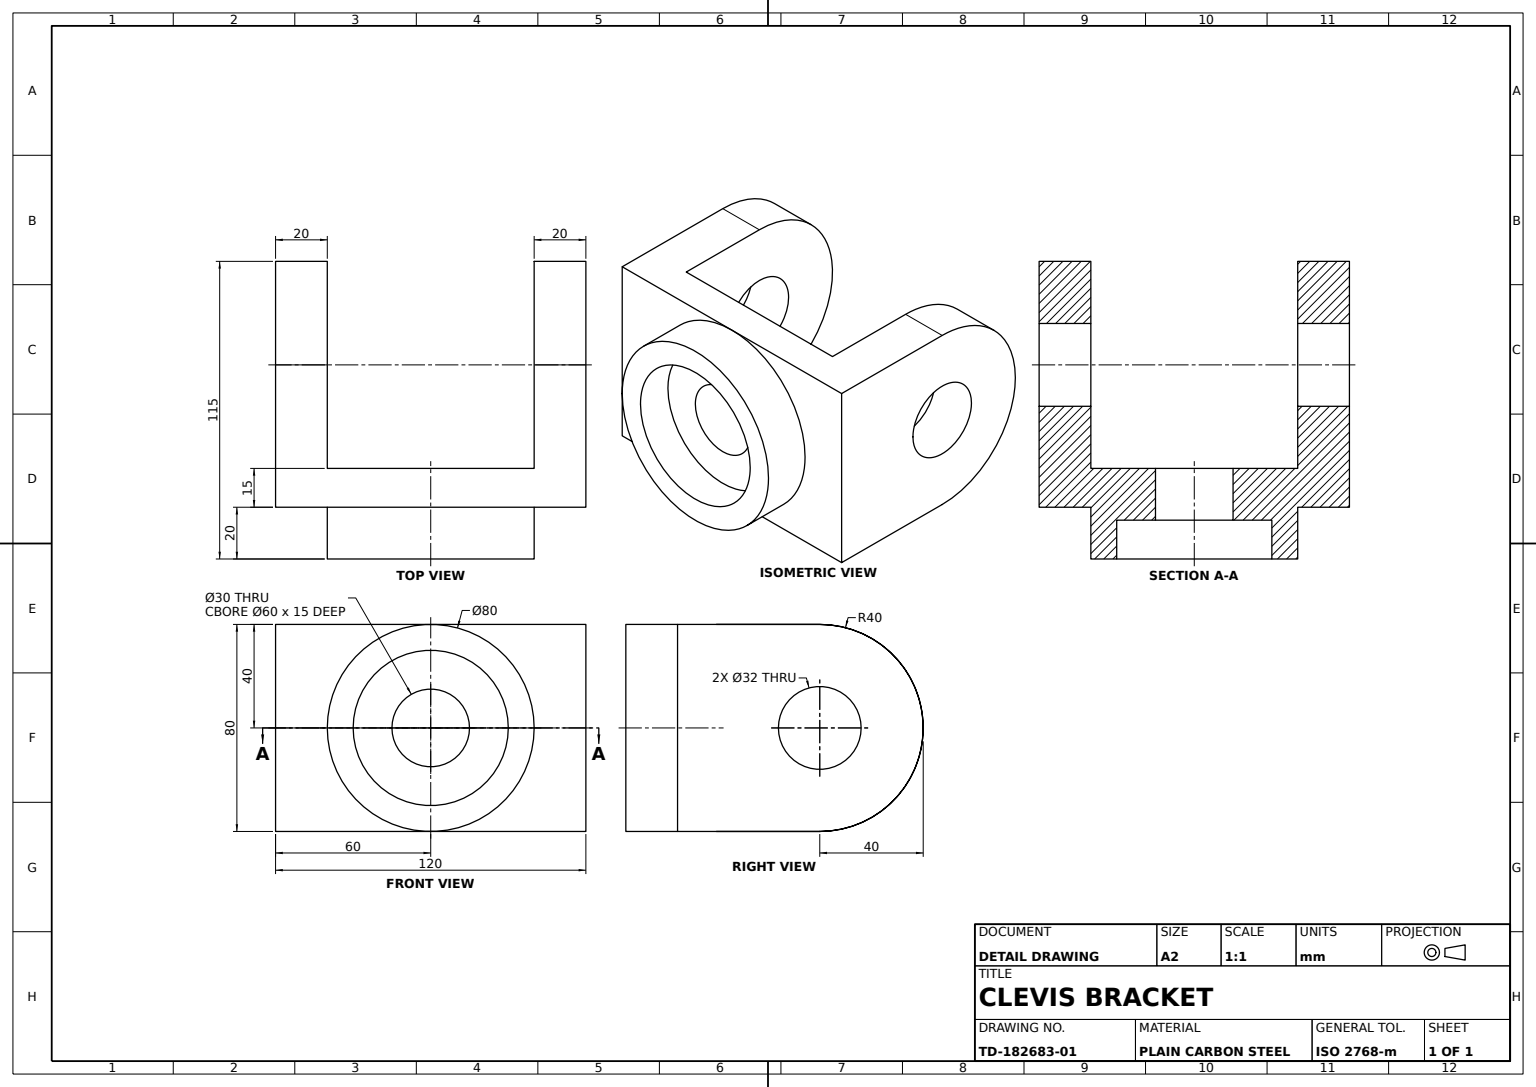
SolidWorks part; units mm, degrees
material "Plain Carbon Steel"
ref_plane "Front Plane" through (0, 0, 0) normal (0, 0, 1) x (1, 0, 0)
ref_plane "Top Plane" through (0, 0, 0) normal (0, 1, 0) x (1, 0, 0)
ref_plane "Right Plane" through (0, 0, 0) normal (1, 0, 0) x (0, 0, -1)
sketch "Base Plate Sketch" plane through (0, 0, 0) normal (0, 0, 1) x (1, 0, 0)
  line L0 (-216.0467, 0) -> (209.0493, 0) construction
  line L1 (0, 118.4321) -> (0, -136.9754) construction
  line L3 (-60, -40) -> (60, -40)
  line L4 (-60, -40) -> (-60, 40)
  line L5 (-60, 40) -> (60, 40)
  line L6 (60, -40) -> (60, 40)
  line L7 (-60, -40) -> (60, 40) construction
  line L8 (-60, 40) -> (60, -40) construction
  point P5 (0, 0)
  dimension "D1" = 120
  dimension "D2" = 80
extrude "Base Plate 120x80x15" add sketch "Base Plate Sketch" along normal blind 15
sketch "Bore Ø30 Sketch" plane through (0, 0, 0) normal (0, 0, -1) x (-1, 0, 0)
  circle A0 centre (0, 0) radius 15
  dimension "D1" = 30
extrude "Bore Ø30" cut sketch "Bore Ø30 Sketch" against normal blind 15
sketch "Hub Boss Sketch" plane through (0, 0, 15) normal (0, 0, 1) x (1, 0, 0)
  circle A0 centre (0, 0) radius 40
  circle A1 centre (0, 0) radius 30
  dimension "D1" = 80
  dimension "D2" = 60
extrude "Hub Boss" add sketch "Hub Boss Sketch" along normal blind 20
sketch "Hub Inner Step Sketch" plane through (0, 0, 15) normal (0, 0, 1) x (1, 0, 0)
  circle A0 centre (0, 0) radius 15
  circle A1 centre (0, 0) radius 30
  circle A2 centre (0, 0) radius 30
  dimension "D2" = 30
  dimension "D1" = 0
extrude "Hub Inner Step" add sketch "Hub Inner Step Sketch" along normal blind 5
sketch "Lug A Sketch" plane through (60, 0, 0) normal (1, 0, 0) x (0, 0, -1)
  line L0 (-66.0023, 0) -> (62.8136, 0) construction
  line L1 (0, -40) -> (0, 40) construction
  line L2 (0, 40) -> (40, 40)
  line L3 (0, -40) -> (40, -40)
  line L5 (0, -40) -> (0, 40)
  circle A0 centre (40, 0) radius 16
  arc A1 (40, -40) -> (40, 40) centre (40, 0) ccw
  dimension "D1" = 80
  dimension "D2" = 32
  dimension "D4" = 40
  dimension "D5" = 80
extrude "Lug A" add sketch "Lug A Sketch" against normal blind 20
sketch "Lug B Sketch" plane through (-60, 0, 0) normal (-1, 0, 0) x (0, 0, 1)
  line L0 (-86.6191, 0) -> (42.8776, 0) construction
  line L1 (-40, 40) -> (15, 40)
  line L2 (-40, -40) -> (15, -40)
  line L3 (15, -40) -> (15, 40) construction
  line L4 (15, -40) -> (15, 40)
  circle A0 centre (-40, 0) radius 16
  arc A1 (-40, 40) -> (-40, -40) centre (-40, 0) ccw
  dimension "D2" = 32
extrude "Lug B" add sketch "Lug B Sketch" against normal blind 20
